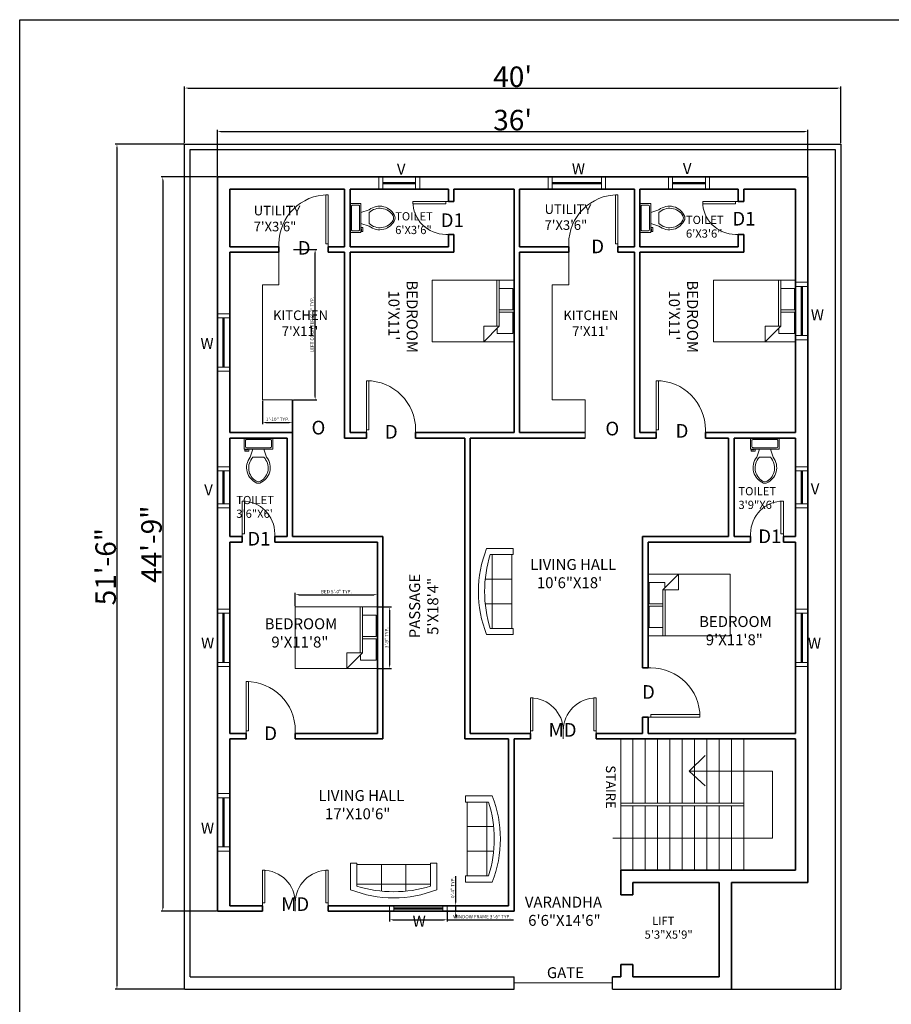
# Model space of a CAD drawing. Units: inches. Extents: x 2169 to 10664, y 1669 to 6352.
# Tile 16 of 17: x 9415 to 10052, y 5632 to 6352. Entities that reach past the tile are written whole.
import ezdxf

# ---------------------------------------------------------------- set-up
doc = ezdxf.new("R2010")
doc.units = ezdxf.units.IN
for name, color, linetype, lineweight in [('A-ANNO-DIMS', 3, 'Continuous', 18), ('A-ANNO-IDEN', 3, 'Continuous', 18), ('A-ANNO-SYMB', 6, 'Continuous', 13), ('A-ANNO-TTLB', 7, 'Continuous', 25), ('A-AREA-IDEN', 4, 'Continuous', 18), ('A-DOOR', 4, 'Continuous', 18), ('A-FLOR-CASE', 8, 'Continuous', 18), ('A-FLOR-FIXT', 9, 'Continuous', 18), ('A-FLOR-STRS', 4, 'Continuous', 18), ('A-FURN', 8, 'Continuous', 18), ('A-GLAZ', 30, 'Continuous', 18), ('A-WALL', 7, 'Continuous', 35), ('C-PROP', 251, 'Continuous', 25)]:
    doc.layers.add(name, color=color, linetype=linetype, lineweight=lineweight)
doc.styles.get("Standard").update_dxf_attribs({"font": 'arial.ttf'})
doc.dimstyles.new('ISO-25', dxfattribs={"dimtxt": 2.5, "dimasz": 2.5, "dimexe": 1.25, "dimexo": 0.625, "dimtad": 1, "dimdec": 0, "dimlunit": 3, "dimtxsty": 'Standard', "dimcen": 2.5, "dimadec": 0, "dimazin": 0, "dimtfac": 1, "dimtdec": 0, "dimtmove": 0, "dimatfit": 3, "dimfxl": 1, "dimarcsym": 0})

# ---------------------------------------------------------------- blocks, each defined once
blk = doc.blocks.new('*U5')
for p, q in [((0, 0), (0, -6)), ((-36, 0), (-36, -6))]:
    blk.add_line(p, q)
blk.add_lwpolyline([(0, 0), (0, 36), (-1.75, 36), (-1.75, 0)], close=True)
blk.add_arc((0, 0), 36, 90, 180)
blk = doc.blocks.new('*U23')
for p, q in [((0, 0), (0, -6)), ((24, 0), (24, -6))]:
    blk.add_line(p, q)
blk.add_lwpolyline([(0, 0), (0, 24), (1.75, 24), (1.75, 0)], close=True)
blk.add_arc((0, 0), 24, 0, 90)
blk = doc.blocks.new('*U22')
for p, q in [((0, 0), (0, -6)), ((36, 0), (36, -6))]:
    blk.add_line(p, q)
blk.add_lwpolyline([(0, 0), (0, 36), (1.75, 36), (1.75, 0)], close=True)
blk.add_arc((0, 0), 36, 0, 90)
blk = doc.blocks.new('*U3')
for p, q in [((-24, 0), (-24, -6)), ((0, 0), (0, -6))]:
    blk.add_line(p, q)
blk.add_lwpolyline([(0, 0), (0, 24), (-1.75, 24), (-1.75, 0)], close=True)
blk.add_arc((0, 0), 24, 90, 180)
blk = doc.blocks.new('*U25')
for p, q in [((0, 0), (0, 6)), ((24, 0), (24, 6))]:
    blk.add_line(p, q)
blk.add_lwpolyline([(0, 0), (0, -24), (1.75, -24), (1.75, 0)], close=True)
blk.add_arc((0, 0), 24, 270, 0)
blk = doc.blocks.new('*U24')
for p, q in [((0, 0), (0, 6)), ((24, 0), (24, 6))]:
    blk.add_line(p, q)
blk.add_lwpolyline([(0, 0), (0, -24), (1.75, -24), (1.75, 0)], close=True)
blk.add_arc((0, 0), 24, 270, 0)
blk = doc.blocks.new('Bed - Queen')
for p, q in [((0, -80.00003), (0, 0)), ((0, 0), (59.99999, 0)), ((59.99999, 0), (59.99999, -80.00003)), ((7.99999, -1.2), (28.79998, -1.2)), ((7.99999, -14.4), (7.99999, -1.2)), ((28.79998, -1.2), (28.79998, -14.4)), ((31.19999, -1.2), (51.99999, -1.2)), ((31.19999, -14.4), (31.19999, -1.2)), ((51.99999, -1.2), (51.99999, -16.4)), ((0, -14.4), (44.8, -14.4)), ((44.8, -16.8), (0, -16.8)), ((59.99999, -29.6), (44.8, -14.4)), ((44.8, -14.4), (44.8, -29.6)), ((51.99999, -16.4), (46.79936, -16.4)), ((44.8, -29.6), (59.99999, -29.6)), ((59.99999, -80.00003), (0, -80.00003))]:
    blk.add_line(p, q)
blk = doc.blocks.new('Sofa - Roundback 7 ft.')
for p, q in [((-12.00002, -32.4421), (-12.00003, -6.5971)), ((11.99997, -32.4421), (11.99998, -6.5971)), ((-36.000027, -34), (-36.000027, -11.4696)), ((-35.999844, -13.3819), (35.9998, -13.3819)), ((35.99998, -34), (35.99998, -11.4696)), ((-36.000027, -32.4421), (35.99998, -32.4421))]:
    blk.add_line(p, q)
for points in [[(-36.000027, -34), (-42.000027, -34), (-42.000027, -8)], [(41.99998, -8), (41.99998, -34), (35.99998, -34)]]:
    blk.add_lwpolyline(points)
for centre, radius, start, end in [((0, -114.25), 114.25, 68.43141, 111.5686), ((-0.00001, -127.1968), 121.1968, 72.72033, 107.2797)]:
    blk.add_arc(centre, radius, start, end)
blk = doc.blocks.new('Toilet - top')
for p, q in [((9.5, -6), (9.5, -2)), ((-10, -8.5), (-8, -8.5)), ((-10, -9.5), (-10, -8.5)), ((-7, -9.5), (-10, -9.5)), ((-8, -8.5), (-8, -8)), ((-7, -8), (-7, -9.5)), ((-4, -8), (-6, -14)), ((4, -14), (-4, -14)), ((4, -8), (6, -14))]:
    blk.add_line(p, q)
blk.add_lwpolyline([(10.5, -8), (10.5, 0), (-10.5, 0), (-10.5, -8)], close=True)
for points in [[(-9.5, -2), (-9.5, -6)], [(8.5, -1), (-8.5, -1)], [(-8.5, -7), (8.5, -7)]]:
    blk.add_lwpolyline(points)
for centre, radius, start, end in [((-8.62, -1.88), 0.884, 81.8699, 188.1301), ((-8.62, -6.12), 0.884, 171.8699, 278.1301), ((8.62, -1.88), 0.884, 351.8699, 98.1301), ((8.62, -6.12), 0.884, 261.8699, 8.1301), ((3.52, -21.58), 12.17, 141.46911, 247.97143), ((4.2, -21.82), 11.33, 136.36773, 238.94682), ((-3.52, -21.58), 12.17, 292.02843, 38.53071), ((-4.2, -21.82), 11.33, 301.05301, 43.63209), ((0, -27.88), 4, 245.73182, 294.26817), ((0, -29), 4, 254.86053, 285.13947)]:
    blk.add_arc(centre, radius, start, end)
blk = doc.blocks.new('*D26')
at = {"layer": 'A-ANNO-DIMS', "color": 0, "lineweight": -2, "transparency": 16777216}
for p, q in [((9559.46, 6237.52), (9559.46, 6271.45)), ((9561.96, 6270.2), (9988.96, 6270.2)), ((9991.46, 6237.52), (9991.46, 6271.45))]:
    blk.add_line(p, q, dxfattribs=at)
at = {"layer": 'A-ANNO-DIMS', "color": 0, "transparency": 16777216}
for points in [[(9561.96, 6270.62), (9561.96, 6269.78), (9559.46, 6270.2)], [(9988.96, 6270.62), (9988.96, 6269.78), (9991.46, 6270.2)]]:
    blk.add_solid(points, dxfattribs=at)
at = {"layer": 'Defpoints', "color": 0, "transparency": 16777216}
for p in [(9991.46, 6270.2), (9559.46, 6236.9), (9991.46, 6236.9)]:
    blk.add_point(p, dxfattribs=at)
at = {"layer": 'A-ANNO-DIMS', "color": 0, "transparency": 16777216, "insert": (9775.46, 6278.49), "char_height": 2.5, "attachment_point": 5}
blk.add_mtext("{\\H6x;36'}", dxfattribs=at)
blk = doc.blocks.new('*D27')
at = {"layer": 'A-ANNO-DIMS', "color": 0, "lineweight": -2, "transparency": 16777216}
for p, q in [((9535.46, 6261.52), (9535.46, 6303.18)), ((9537.96, 6301.93), (10012.96, 6301.93)), ((10015.46, 6261.52), (10015.46, 6303.18))]:
    blk.add_line(p, q, dxfattribs=at)
at = {"layer": 'A-ANNO-DIMS', "color": 0, "transparency": 16777216}
for points in [[(9537.96, 6302.34), (9537.96, 6301.51), (9535.46, 6301.93)], [(10012.96, 6302.34), (10012.96, 6301.51), (10015.46, 6301.93)]]:
    blk.add_solid(points, dxfattribs=at)
at = {"layer": 'Defpoints', "color": 0, "transparency": 16777216}
for p in [(10015.46, 6301.93), (9535.46, 6260.9), (10015.46, 6260.9)]:
    blk.add_point(p, dxfattribs=at)
at = {"layer": 'A-ANNO-DIMS', "color": 0, "transparency": 16777216, "insert": (9775.46, 6310.21), "char_height": 2.5, "attachment_point": 5}
blk.add_mtext("{\\H6x;40'}", dxfattribs=at)
blk = doc.blocks.new('*D28')
at = {"layer": 'A-ANNO-DIMS', "color": 0, "lineweight": -2, "transparency": 16777216}
for p, q in [((9558.84, 6236.9), (9518.24, 6236.9)), ((9519.49, 6234.4), (9519.49, 5702.4)), ((9558.84, 5699.9), (9518.24, 5699.9))]:
    blk.add_line(p, q, dxfattribs=at)
at = {"layer": 'A-ANNO-DIMS', "color": 0, "transparency": 16777216}
for points in [[(9519.08, 6234.4), (9519.91, 6234.4), (9519.49, 6236.9)], [(9519.08, 5702.4), (9519.91, 5702.4), (9519.49, 5699.9)]]:
    blk.add_solid(points, dxfattribs=at)
at = {"layer": 'Defpoints', "color": 0, "transparency": 16777216}
for p in [(9559.46, 6236.9), (9519.49, 5699.9), (9559.46, 5699.9)]:
    blk.add_point(p, dxfattribs=at)
at = {"layer": 'A-ANNO-DIMS', "color": 0, "transparency": 16777216, "insert": (9511.21, 5968.31), "char_height": 2.5, "attachment_point": 5, "rotation": 90}
blk.add_mtext('{\\H6x;44\'-9"}', dxfattribs=at)
blk = doc.blocks.new('*D29')
at = {"layer": 'A-ANNO-DIMS', "color": 0, "lineweight": -2, "transparency": 16777216}
for p, q in [((9534.84, 6260.9), (9484.72, 6260.9)), ((9485.97, 6258.4), (9485.97, 5645.4)), ((9534.84, 5642.9), (9484.72, 5642.9))]:
    blk.add_line(p, q, dxfattribs=at)
at = {"layer": 'A-ANNO-DIMS', "color": 0, "transparency": 16777216}
for points in [[(9485.56, 6258.4), (9486.39, 6258.4), (9485.97, 6260.9)], [(9485.56, 5645.4), (9486.39, 5645.4), (9485.97, 5642.9)]]:
    blk.add_solid(points, dxfattribs=at)
at = {"layer": 'Defpoints', "color": 0, "transparency": 16777216}
for p in [(9535.46, 6260.9), (9485.97, 5642.9), (9535.46, 5642.9)]:
    blk.add_point(p, dxfattribs=at)
at = {"layer": 'A-ANNO-DIMS', "color": 0, "transparency": 16777216, "insert": (9477.69, 5951.9), "char_height": 2.5, "attachment_point": 5, "rotation": 90}
blk.add_mtext('{\\H6x;51\'-6"}', dxfattribs=at)
blk = doc.blocks.new('WIN-36-WALL-9')
for p, q in [((9, 42), (0, 42)), ((9, 39), (0, 39)), ((4, 39), (4, 3)), ((4.5, 39), (4.5, 3)), ((5, 39), (5, 3)), ((9, 3), (0, 3)), ((9, 0), (0, 0))]:
    blk.add_line(p, q)
blk = doc.blocks.new('WIN-24-WALL-9')
for p, q in [((9, 30), (0, 30)), ((9, 27), (0, 27)), ((4, 27), (4, 3)), ((4.5, 27), (4.5, 3)), ((5, 27), (5, 3)), ((9, 3), (0, 3)), ((9, 0), (0, 0))]:
    blk.add_line(p, q)
blk = doc.blocks.new('WIN-36-WALL-4')
for p, q in [((0, 4), (0, 0)), ((3, 4), (3, 0)), ((3, 2.5), (39, 2.5)), ((3, 2), (39, 2)), ((3, 1.5), (39, 1.5)), ((39, 4), (39, 0)), ((42, 4), (42, 0))]:
    blk.add_line(p, q)
blk = doc.blocks.new('STAIR-DOGLEG-PLAN')
for p, q in [((0, 0), (0, 96)), ((9, 49), (9, 96)), ((18, 49), (18, 96)), ((27, 49), (27, 96)), ((36, 49), (36, 96)), ((45, 49), (45, 96)), ((54, 49), (54, 96)), ((63, 49), (63, 96)), ((72, 49), (72, 96)), ((81, 49), (81, 96)), ((90, 0), (90, 96)), ((90, 49), (0, 49)), ((90, 47), (0, 47)), ((9, 0), (9, 47)), ((18, 0), (18, 47)), ((27, 0), (27, 47)), ((36, 0), (36, 47)), ((45, 0), (45, 47)), ((54, 0), (54, 47)), ((63, 0), (63, 47)), ((72, 0), (72, 47)), ((81, 0), (81, 47))]:
    blk.add_line(p, q)
blk = doc.blocks.new('STAIR-DIRECTION')
for p, q in [((55.67, 49), (67.5, 60.35)), ((116.68, 49), (55.67, 49)), ((55.67, 49), (67.5, 38.08)), ((116.68, 0), (116.68, 49)), ((0, 0), (116.68, 0))]:
    blk.add_line(p, q)
blk = doc.blocks.new('COUNTER-UTILITY-L')
for p, q in [((12, 110), (12, 84)), ((0, 0), (0, 84)), ((0, 84), (12, 84)), ((0, 0), (22, 0))]:
    blk.add_line(p, q)
blk = doc.blocks.new('COUNTER-UTILITY-R')
for p, q in [((12, 136), (12, 112)), ((0, 28), (0, 112)), ((0, 112), (12, 112)), ((0, 28), (24, 28)), ((24, 0), (24, 28))]:
    blk.add_line(p, q)
blk = doc.blocks.new('*D55')
at = {"layer": 'A-ANNO-DIMS', "color": 0, "lineweight": -2, "transparency": 16777216}
for p, q in [((9616.46, 5923.02), (9616.46, 5932.65)), ((9618.96, 5931.4), (9673.96, 5931.4)), ((9676.46, 5923.02), (9676.46, 5932.65))]:
    blk.add_line(p, q, dxfattribs=at)
at = {"layer": 'A-ANNO-DIMS', "color": 0, "transparency": 16777216}
for points in [[(9618.96, 5931.81), (9618.96, 5930.98), (9616.46, 5931.4)], [(9673.96, 5931.81), (9673.96, 5930.98), (9676.46, 5931.4)]]:
    blk.add_solid(points, dxfattribs=at)
at = {"layer": 'Defpoints', "color": 0, "transparency": 16777216}
for p in [(9676.46, 5931.4), (9616.46, 5922.4), (9676.46, 5922.4)]:
    blk.add_point(p, dxfattribs=at)
at = {"layer": 'A-ANNO-DIMS', "color": 0, "transparency": 16777216, "insert": (9646.46, 5933.3), "char_height": 2.5, "attachment_point": 5}
blk.add_mtext('BED 5\'-0" TYP.', dxfattribs=at)
blk = doc.blocks.new('*D56')
at = {"layer": 'A-ANNO-DIMS', "color": 0, "lineweight": -2, "transparency": 16777216}
for p, q in [((9677.09, 5922.4), (9686.71, 5922.4)), ((9685.46, 5919.9), (9685.46, 5879.9)), ((9677.09, 5877.4), (9686.71, 5877.4))]:
    blk.add_line(p, q, dxfattribs=at)
at = {"layer": 'A-ANNO-DIMS', "color": 0, "transparency": 16777216}
for points in [[(9685.05, 5919.9), (9685.88, 5919.9), (9685.46, 5922.4)], [(9685.05, 5879.9), (9685.88, 5879.9), (9685.46, 5877.4)]]:
    blk.add_solid(points, dxfattribs=at)
at = {"layer": 'Defpoints', "color": 0, "transparency": 16777216}
for p in [(9676.46, 5922.4), (9676.46, 5877.4), (9685.46, 5877.4)]:
    blk.add_point(p, dxfattribs=at)
at = {"layer": 'A-ANNO-DIMS', "color": 0, "transparency": 16777216, "insert": (9683.56, 5899.9), "char_height": 2.5, "attachment_point": 5, "rotation": 90}
blk.add_mtext('3\'-9" TYP.', dxfattribs=at)
blk = doc.blocks.new('*D75')
at = {"layer": 'A-ANNO-DIMS', "color": 0, "lineweight": -2, "transparency": 16777216}
for p, q in [((9685.46, 5699.27), (9685.46, 5692.35)), ((9727.46, 5699.27), (9727.46, 5692.35)), ((9687.96, 5693.6), (9724.96, 5693.6)), ((9727.46, 5693.6), (9776.04, 5693.6))]:
    blk.add_line(p, q, dxfattribs=at)
at = {"layer": 'A-ANNO-DIMS', "color": 0, "transparency": 16777216}
for points in [[(9687.96, 5694.01), (9687.96, 5693.18), (9685.46, 5693.6)], [(9724.96, 5694.01), (9724.96, 5693.18), (9727.46, 5693.6)]]:
    blk.add_solid(points, dxfattribs=at)
at = {"layer": 'Defpoints', "color": 0, "transparency": 16777216}
for p in [(9685.46, 5699.9), (9727.46, 5699.9), (9727.46, 5693.6)]:
    blk.add_point(p, dxfattribs=at)
at = {"layer": 'A-ANNO-DIMS', "color": 0, "transparency": 16777216, "insert": (9753, 5695.52), "char_height": 2.5, "attachment_point": 5}
blk.add_mtext('WINDOW FRAME 3\'-6" TYP.', dxfattribs=at)
blk = doc.blocks.new('*D76')
at = {"layer": 'A-ANNO-DIMS', "color": 0, "lineweight": -2, "transparency": 16777216}
for p, q in [((9733.76, 5706.4), (9733.76, 5725.39)), ((9728.09, 5703.9), (9735.01, 5703.9)), ((9733.76, 5699.9), (9733.76, 5703.9)), ((9728.09, 5699.9), (9735.01, 5699.9)), ((9733.76, 5697.4), (9733.76, 5694.9))]:
    blk.add_line(p, q, dxfattribs=at)
at = {"layer": 'A-ANNO-DIMS', "color": 0, "transparency": 16777216}
for points in [[(9733.35, 5706.4), (9734.18, 5706.4), (9733.76, 5703.9)], [(9733.35, 5697.4), (9734.18, 5697.4), (9733.76, 5699.9)]]:
    blk.add_solid(points, dxfattribs=at)
at = {"layer": 'Defpoints', "color": 0, "transparency": 16777216}
for p in [(9727.46, 5703.9), (9733.76, 5703.9), (9727.46, 5699.9)]:
    blk.add_point(p, dxfattribs=at)
at = {"layer": 'A-ANNO-DIMS', "color": 0, "transparency": 16777216, "insert": (9731.86, 5717.14), "char_height": 2.5, "attachment_point": 5, "rotation": 90}
blk.add_mtext('0\'-4" TYP.', dxfattribs=at)
blk = doc.blocks.new('*D81')
at = {"layer": 'A-ANNO-DIMS', "color": 0, "lineweight": -2, "transparency": 16777216}
for p, q in [((9615.09, 6183.9), (9632.21, 6183.9)), ((9630.96, 6076.4), (9630.96, 6181.4)), ((9615.09, 6073.9), (9632.21, 6073.9))]:
    blk.add_line(p, q, dxfattribs=at)
at = {"layer": 'A-ANNO-DIMS', "color": 0, "transparency": 16777216}
for points in [[(9630.55, 6181.4), (9631.38, 6181.4), (9630.96, 6183.9)], [(9630.55, 6076.4), (9631.38, 6076.4), (9630.96, 6073.9)]]:
    blk.add_solid(points, dxfattribs=at)
at = {"layer": 'Defpoints', "color": 0, "transparency": 16777216}
for p in [(9614.46, 6183.9), (9630.96, 6183.9), (9614.46, 6073.9)]:
    blk.add_point(p, dxfattribs=at)
at = {"layer": 'A-ANNO-DIMS', "color": 0, "transparency": 16777216, "insert": (9629.04, 6128.9), "char_height": 2.5, "attachment_point": 5, "rotation": 90}
blk.add_mtext('LEFT COUNTER 9\'-2" TYP.', dxfattribs=at)
blk = doc.blocks.new('*D82')
at = {"layer": 'A-ANNO-DIMS', "color": 0, "lineweight": -2, "transparency": 16777216}
for p, q in [((9592.46, 6073.27), (9592.46, 6056.15)), ((9614.46, 6073.27), (9614.46, 6056.15)), ((9594.96, 6057.4), (9611.96, 6057.4))]:
    blk.add_line(p, q, dxfattribs=at)
at = {"layer": 'A-ANNO-DIMS', "color": 0, "transparency": 16777216}
for points in [[(9594.96, 6057.81), (9594.96, 6056.98), (9592.46, 6057.4)], [(9611.96, 6057.81), (9611.96, 6056.98), (9614.46, 6057.4)]]:
    blk.add_solid(points, dxfattribs=at)
at = {"layer": 'Defpoints', "color": 0, "transparency": 16777216}
for p in [(9592.46, 6073.9), (9614.46, 6073.9), (9614.46, 6057.4)]:
    blk.add_point(p, dxfattribs=at)
at = {"layer": 'A-ANNO-DIMS', "color": 0, "transparency": 16777216, "insert": (9603.46, 6059.3), "char_height": 2.5, "attachment_point": 5}
blk.add_mtext('1\'-10" TYP.', dxfattribs=at)

msp = doc.modelspace()

# ---------------------------------------------------------------- linework, layer by layer
at = {"layer": 'A-ANNO-TTLB'}
msp.add_lwpolyline([(9414.82, 6351.94), (10664.28, 6351.94), (10664.28, 5158.92), (9414.82, 5158.92)], close=True, dxfattribs=at)
at = {"layer": 'A-DOOR'}
msp.add_line((9776.46, 5647.4), (9848.46, 5647.4), dxfattribs=at)
at = {"layer": 'A-WALL'}
for p, q in [((9559.46, 6236.9), (9991.46, 6236.9)), ((9559.46, 5699.9), (9559.46, 6236.9)), ((9991.46, 6236.9), (9991.46, 5720.9)), ((9568.46, 6227.9), (9652.46, 6227.9)), ((9568.46, 6185.9), (9568.46, 6227.9)), ((9652.46, 6185.9), (9652.46, 6227.9)), ((9656.46, 6227.9), (9728.46, 6227.9)), ((9656.46, 6185.9), (9656.46, 6227.9)), ((9728.46, 6218.9), (9728.46, 6227.9)), ((9732.46, 6227.9), (9776.46, 6227.9)), ((9732.46, 6218.9), (9732.46, 6227.9)), ((9776.46, 6049.9), (9776.46, 6227.9)), ((9780.46, 6227.9), (9864.46, 6227.9)), ((9780.46, 6185.9), (9780.46, 6227.9)), ((9864.46, 6185.9), (9864.46, 6227.9)), ((9868.46, 6227.9), (9940.46, 6227.9)), ((9868.46, 6185.9), (9868.46, 6227.9)), ((9940.46, 6218.9), (9940.46, 6227.9)), ((9944.46, 6227.9), (9982.46, 6227.9)), ((9944.46, 6218.9), (9944.46, 6227.9)), ((9982.46, 6227.9), (9982.46, 6049.9)), ((9728.46, 6218.9), (9732.46, 6218.9)), ((9940.46, 6218.9), (9944.46, 6218.9)), ((9728.46, 6185.9), (9728.46, 6194.9)), ((9728.46, 6194.9), (9732.46, 6194.9)), ((9732.46, 6181.9), (9732.46, 6194.9)), ((9940.46, 6185.9), (9940.46, 6194.9)), ((9940.46, 6194.9), (9944.46, 6194.9)), ((9944.46, 6181.9), (9944.46, 6194.9)), ((9568.46, 6185.9), (9604.46, 6185.9)), ((9568.46, 6181.9), (9604.46, 6181.9)), ((9568.46, 6049.9), (9568.46, 6181.9)), ((9604.46, 6181.9), (9604.46, 6185.9)), ((9640.46, 6185.9), (9652.46, 6185.9)), ((9640.46, 6181.9), (9640.46, 6185.9)), ((9640.46, 6181.9), (9652.46, 6181.9)), ((9652.46, 6045.9), (9652.46, 6181.9)), ((9656.46, 6185.9), (9728.46, 6185.9)), ((9656.46, 6181.9), (9732.46, 6181.9)), ((9656.46, 6049.9), (9656.46, 6181.9)), ((9780.46, 6185.9), (9816.46, 6185.9)), ((9780.46, 6181.9), (9816.46, 6181.9)), ((9780.46, 6049.9), (9780.46, 6181.9)), ((9816.46, 6181.9), (9816.46, 6185.9)), ((9852.46, 6185.9), (9864.46, 6185.9)), ((9852.46, 6181.9), (9852.46, 6185.9)), ((9852.46, 6181.9), (9864.46, 6181.9)), ((9864.46, 6045.9), (9864.46, 6181.9)), ((9868.46, 6185.9), (9940.46, 6185.9)), ((9868.46, 6181.9), (9944.46, 6181.9)), ((9868.46, 6049.9), (9868.46, 6181.9)), ((9614.46, 5973.9), (9614.46, 6073.9)), ((9568.46, 6049.9), (9614.46, 6049.9)), ((9656.46, 6049.9), (9668.46, 6049.9)), ((9668.46, 6045.9), (9668.46, 6049.9)), ((9704.46, 6049.9), (9776.46, 6049.9)), ((9704.46, 6045.9), (9704.46, 6049.9)), ((9780.46, 6049.9), (9828.46, 6049.9)), ((9868.46, 6049.9), (9880.46, 6049.9)), ((9880.46, 6045.9), (9880.46, 6049.9)), ((9916.46, 6049.9), (9982.46, 6049.9)), ((9916.46, 6045.9), (9916.46, 6049.9)), ((9568.46, 6045.9), (9610.46, 6045.9)), ((9568.46, 5973.9), (9568.46, 6045.9)), ((9610.46, 5973.9), (9610.46, 6045.9)), ((9652.46, 6045.9), (9668.46, 6045.9)), ((9704.46, 6045.9), (9740.46, 6045.9)), ((9740.46, 5825.9), (9740.46, 6045.9)), ((9744.46, 6045.9), (9828.46, 6045.9)), ((9744.46, 5829.9), (9744.46, 6045.9)), ((9864.46, 6045.9), (9880.46, 6045.9)), ((9916.46, 6045.9), (9933.46, 6045.9)), ((9933.46, 6045.9), (9933.46, 5973.9)), ((9937.46, 6045.9), (9982.46, 6045.9)), ((9937.46, 6045.9), (9937.46, 5973.9)), ((9982.46, 6045.9), (9982.46, 5973.9)), ((9568.46, 5973.9), (9577.46, 5973.9)), ((9577.46, 5969.9), (9577.46, 5973.9)), ((9601.46, 5973.9), (9610.46, 5973.9)), ((9601.46, 5969.9), (9601.46, 5973.9)), ((9614.46, 5973.9), (9680.46, 5973.9)), ((9680.46, 5825.9), (9680.46, 5973.9)), ((9870.46, 5973.9), (9933.46, 5973.9)), ((9870.46, 5973.9), (9870.46, 5877.9)), ((9937.46, 5973.9), (9949.46, 5973.9)), ((9949.46, 5973.9), (9949.46, 5969.9)), ((9973.46, 5973.9), (9982.46, 5973.9)), ((9973.46, 5973.9), (9973.46, 5969.9)), ((9568.46, 5969.9), (9577.46, 5969.9)), ((9568.46, 5829.9), (9568.46, 5969.9)), ((9601.46, 5969.9), (9676.46, 5969.9)), ((9676.46, 5829.9), (9676.46, 5969.9)), ((9874.46, 5969.9), (9949.46, 5969.9)), ((9874.46, 5969.9), (9874.46, 5877.9)), ((9973.46, 5969.9), (9982.46, 5969.9)), ((9982.46, 5969.9), (9982.46, 5829.9)), ((9870.46, 5877.9), (9874.46, 5877.9)), ((9870.46, 5841.9), (9874.46, 5841.9)), ((9870.46, 5841.9), (9870.46, 5829.9)), ((9874.46, 5841.9), (9874.46, 5829.9)), ((9568.46, 5829.9), (9580.46, 5829.9)), ((9580.46, 5825.9), (9580.46, 5829.9)), ((9616.46, 5829.9), (9676.46, 5829.9)), ((9616.46, 5825.9), (9616.46, 5829.9)), ((9744.46, 5829.9), (9788.46, 5829.9)), ((9788.46, 5825.9), (9788.46, 5829.9)), ((9836.46, 5829.9), (9870.46, 5829.9)), ((9836.46, 5825.9), (9836.46, 5829.9)), ((9874.46, 5829.9), (9982.46, 5829.9)), ((9568.46, 5825.9), (9580.46, 5825.9)), ((9568.46, 5703.9), (9568.46, 5825.9)), ((9616.46, 5825.9), (9680.46, 5825.9)), ((9740.46, 5825.9), (9772.46, 5825.9)), ((9772.46, 5703.9), (9772.46, 5825.9)), ((9776.46, 5825.9), (9788.46, 5825.9)), ((9776.46, 5699.9), (9776.46, 5825.9)), ((9836.46, 5825.9), (9982.46, 5825.9)), ((9982.46, 5825.9), (9982.46, 5729.9)), ((9982.46, 5729.9), (9854.46, 5729.9)), ((9854.46, 5711.9), (9854.46, 5729.9)), ((9926.46, 5720.9), (9863.46, 5720.9)), ((9863.46, 5711.9), (9863.46, 5720.9)), ((9926.46, 5651.9), (9926.46, 5720.9)), ((9991.46, 5720.9), (9935.46, 5720.9)), ((9935.46, 5642.9), (9935.46, 5720.9)), ((9863.46, 5711.9), (9854.46, 5711.9)), ((9592.46, 5703.9), (9568.46, 5703.9)), ((9592.46, 5699.9), (9592.46, 5703.9)), ((9772.46, 5703.9), (9640.46, 5703.9)), ((9640.46, 5699.9), (9640.46, 5703.9)), ((9592.46, 5699.9), (9559.46, 5699.9)), ((9776.46, 5699.9), (9640.46, 5699.9)), ((9854.46, 5651.9), (9854.46, 5660.9)), ((9854.46, 5660.9), (9863.46, 5660.9)), ((9863.46, 5651.9), (9863.46, 5660.9)), ((9848.46, 5651.9), (9854.46, 5651.9)), ((9863.46, 5651.9), (9926.46, 5651.9))]:
    msp.add_line(p, q, dxfattribs=at)
at = {"layer": 'C-PROP'}
for p, q in [((9535.46, 6260.9), (10015.46, 6260.9)), ((9535.46, 5642.9), (9535.46, 6260.9)), ((10015.46, 6260.9), (10015.46, 5642.9)), ((9539.46, 6256.9), (10011.46, 6256.9)), ((9539.46, 5651.9), (9539.46, 6256.9)), ((10011.46, 6256.9), (10011.46, 5642.9)), ((9539.46, 5651.9), (9776.46, 5651.9)), ((9776.46, 5642.9), (9776.46, 5651.9)), ((9848.46, 5642.9), (9848.46, 5651.9)), ((9535.46, 5642.9), (9776.46, 5642.9)), ((9848.46, 5642.9), (9935.46, 5642.9)), ((9935.46, 5642.9), (10015.46, 5642.9))]:
    msp.add_line(p, q, dxfattribs=at)

# ---------------------------------------------------------------- block references
at = {"layer": 'A-ANNO-SYMB'}
msp.add_blockref('STAIR-DIRECTION', (9848.79, 5753.4), dxfattribs=at)
at = {"layer": 'A-DOOR'}
for name, p in [('*U5', (9640.46, 6187.9)), ('*U5', (9852.46, 6187.9)), ('*U22', (9668.46, 6051.9)), ('*U22', (9880.46, 6051.9)), ('*U23', (9577.46, 5975.9)), ('*U3', (9973.46, 5975.9)), ('*U22', (9580.46, 5831.9)), ('*U23', (9788.46, 5831.9)), ('*U3', (9836.46, 5831.9)), ('*U23', (9592.46, 5705.9)), ('*U3', (9640.46, 5705.9))]:
    msp.add_blockref(name, p, dxfattribs=at)
at = {"layer": 'A-DOOR', "rotation": 270}
for name, p in [('*U24', (9726.46, 6218.9)), ('*U25', (9938.46, 6218.9)), ('*U5', (9876.46, 5841.9))]:
    msp.add_blockref(name, p, dxfattribs=at)
at = {"layer": 'A-FLOR-CASE'}
for name, p in [('COUNTER-UTILITY-L', (9592.46, 6073.9)), ('COUNTER-UTILITY-R', (9804.46, 6045.9))]:
    msp.add_blockref(name, p, dxfattribs=at)
at = {"layer": 'A-FLOR-FIXT', "rotation": 90}
for p in [(9656.46, 6206.9), (9868.46, 6206.9)]:
    msp.add_blockref('Toilet - top', p, dxfattribs=at)
at = {"layer": 'A-FLOR-FIXT'}
for p in [(9589.46, 6045.9), (9959.96, 6045.9)]:
    msp.add_blockref('Toilet - top', p, dxfattribs=at)
at = {"layer": 'A-FLOR-STRS'}
msp.add_blockref('STAIR-DOGLEG-PLAN', (9854.46, 5729.9), dxfattribs=at)
at = {"layer": 'A-FURN', "xscale": 0.75, "yscale": 0.75, "zscale": 0.75}
for name, p, rotation in [('Bed - Queen', (9776.46, 6161.4), 270), ('Bed - Queen', (9982.46, 6161.4), 270), ('Sofa - Roundback 7 ft.', (9750.42, 5933.68), 89.99999999999999), ('Bed - Queen', (9874.46, 5901.4), 89.99999999999999), ('Bed - Queen', (9676.46, 5922.4), 270), ('Sofa - Roundback 7 ft.', (9766.49, 5752.74), 270), ('Sofa - Roundback 7 ft.', (9688.42, 5709.62), 180)]:
    msp.add_blockref(name, p, dxfattribs=dict(at, rotation=rotation))
at = {"layer": 'A-GLAZ'}
for name, p, rotation in [('WIN-24-WALL-9', (9707.46, 6227.9), 89.9999999999965), ('WIN-36-WALL-9', (9801.46, 6236.9), 269.9999999999998), ('WIN-24-WALL-9', (9889.46, 6236.9), 270.0000000000003), ('WIN-24-WALL-9', (9568.46, 6024.9), 180), ('WIN-24-WALL-9', (9991.46, 6024.9), 180)]:
    msp.add_blockref(name, p, dxfattribs=dict(at, rotation=rotation))
for name, p in [('WIN-36-WALL-9', (9982.46, 6117.9)), ('WIN-36-WALL-9', (9559.46, 6094.9)), ('WIN-36-WALL-9', (9559.46, 5878.9)), ('WIN-36-WALL-9', (9982.46, 5878.9)), ('WIN-36-WALL-9', (9559.46, 5743.9)), ('WIN-36-WALL-4', (9685.46, 5699.9))]:
    msp.add_blockref(name, p, dxfattribs=at)

# ---------------------------------------------------------------- texts
at = {"layer": 'A-ANNO-IDEN', "attachment_point": 1}
for s, heights, insert, char_height in [('V', [8.65], (9690.78, 6246.71), 8), ('W', [8.65], (9818.77, 6246.94), 8), ('V', [8.65], (9900, 6247.05), 8), ('D1', [0], (9722.82, 6210.27), 10), ('D1', [0], (9936.16, 6211.38), 10), ('D', [0], (9618.17, 6190.08), 10), ('D', [0], (9832.93, 6191.13), 10), ('W', [8.65], (9993.59, 6140.13), 8), ('W', [8.65], (9547.09, 6119.19), 8), ('O', [8.65], (9628.3, 6058.58), 10), ('O', [8.65], (9843.27, 6057.89), 10), ('D', [0], (9681.96, 6055.52), 10), ('D', [0], (9894.64, 6056.19), 10), ('V', [8.65], (9549.81, 6012.07), 8), ('V', [8.65], (9993.53, 6012.74), 8), ('D1', [0], (9581.35, 5977.32), 10), ('D1', [0], (9955.12, 5979.07), 10), ('W', [8.65], (9547.52, 5900.03), 8), ('W', [8.65], (9991.46, 5899.85), 8), ('D', [0], (9870.07, 5865.22), 10), ('D', [0], (9593.71, 5834.99), 10), ('MD', [8.65], (9801.72, 5837.48), 10), ('W', [8.65], (9547.43, 5764.66), 8), ('MD', [8.65], (9606.12, 5710.07), 10), ('W', [8.65], (9702.27, 5696.56), 8)]:
    msp.add_mtext_dynamic_manual_height_columns(s, width=418.9353, gutter_width=12.5, heights=heights, dxfattribs=dict(at, insert=insert, char_height=char_height))
at = {"layer": 'A-AREA-IDEN', "attachment_point": 1}
for s, width, insert, char_height in [('UTILITY\\P7\'X3\'6"', 378.2909, (9586, 6215.8), 7), ('UTILITY\\P7\'X3\'6"', 378.2909, (9798.79, 6216.87), 7), ('TOILET\\P6\'X3\'6"', 229.0681, (9689.5, 6211.14), 6), ('TOILET\\P6\'X3\'6"', 229.0681, (9902.22, 6208.52), 6), ("KITCHEN\\P   7'X11'", 624.2169, (9600.12, 6139.26), 7), ("KITCHEN\\P   7'X11'", 624.2169, (9812.57, 6139.23), 7), ('TOILET\\P3\'9"X6\'', 181.098, (9940.61, 6010.09), 6), ('TOILET\\P3\'6"X6\'', 181.098, (9573.29, 6003.61), 6), ('LIVING HALL\\P  10\'6"X18\'', 560.0068, (9788.29, 5957.48), 8), ('BEDROOM\\P  9\'X11\'8"', 585.4842, (9594.05, 5914.09), 8), ('BEDROOM\\P  9\'X11\'8"', 585.4842, (9911.86, 5915.74), 8), ('LIVING HALL\\P  17\'X10\'6"', 430.6105, (9633.29, 5788.47), 8), ('VARANDHA\\P 6\'6"X14\'6"', 244.2229, (9784.37, 5710.52), 8), ('   LIFT\\P5\'3"X5\'9"', 367.579, (9871.98, 5695.77), 6), ('GATE', 121.9604, (9800.51, 5658.92), 8)]:
    msp.add_mtext_dynamic_manual_height_columns(s, width=width, gutter_width=12.5, heights=[0], dxfattribs=dict(at, insert=insert, char_height=char_height))
for s, width, insert, char_height, rotation in [("BEDROOM\\P   10'X11'", 613.8035, (9705.93, 6161.25), 8, 270), ("BEDROOM\\P   10'X11'", 613.8035, (9911.06, 6161.25), 8, 270), ('PASSAGE\\P 5\'X18\'4"', 733.7273, (9699.75, 5899.53), 8, 90), ('STAIRE', 319.0814, (9850.7, 5806.57), 7, 270)]:
    msp.add_mtext_dynamic_manual_height_columns(s, width=width, gutter_width=12.5, heights=[0], dxfattribs=dict(at, insert=insert, char_height=char_height, rotation=rotation))

# ---------------------------------------------------------------- dimensions: what is measured, and where the dimension line sits
at = {"layer": 'A-ANNO-DIMS'}
for base, p1, p2, text, override, picture, middle in [((10015.46, 6301.93), (9535.46, 6260.9), (10015.46, 6260.9), '{\\H6x;<>}', {"dimclrd": 0, "dimclre": 0, "dimclrt": 0}, '*D27', (9775.46, 6310.21)), ((9614.46, 6057.4), (9592.46, 6073.9), (9614.46, 6073.9), '<> TYP.', {"dimdec": 1, "dimlfac": 1, "dimrnd": 0, "dimzin": 1, "dimdsep": 46, "dimlunit": 4, "dimfrac": 2}, '*D82', (9603.46, 6059.3)), ((9676.46, 5931.4), (9616.46, 5922.4), (9676.46, 5922.4), 'BED <> TYP.', {"dimdec": 1, "dimlfac": 1, "dimrnd": 0, "dimzin": 1, "dimdsep": 46, "dimlunit": 4, "dimfrac": 2}, '*D55', (9646.46, 5933.3)), ((9727.46, 5693.6), (9685.46, 5699.9), (9727.46, 5699.9), 'WINDOW FRAME <> TYP.', {"dimdec": 1, "dimlfac": 1, "dimrnd": 0, "dimzin": 1, "dimdsep": 46, "dimlunit": 4, "dimfrac": 2}, '*D75', (9753, 5695.52))]:
    dim = msp.add_linear_dim(base=base, p1=p1, p2=p2, text=text, dimstyle='ISO-25', override=override, dxfattribs=at)
    dim.commit()
    dim.dimension.update_dxf_attribs({"geometry": picture, "text_midpoint": middle})
dim = msp.add_linear_dim(base=(9991.46, 6270.2), p1=(9559.46, 6236.9), p2=(9991.46, 6236.9), text='{\\H6x;<>}', dimstyle='ISO-25', override={"dimclrd": 0, "dimclre": 0, "dimclrt": 0}, dxfattribs=at)
dim.commit()
dim.dimension.update_dxf_attribs({"geometry": '*D26', "text_midpoint": (9775.46, 6270.2), "dimtype": 160})
for base, p1, p2, picture, middle in [((9485.97, 5642.9), (9535.46, 6260.9), (9535.46, 5642.9), '*D29', (9485.97, 5951.9)), ((9519.49, 5699.9), (9559.46, 6236.9), (9559.46, 5699.9), '*D28', (9519.49, 5968.31))]:
    dim = msp.add_linear_dim(base=base, p1=p1, p2=p2, angle=90, text='{\\H6x;<>}', dimstyle='ISO-25', override={"dimclrd": 0, "dimclre": 0, "dimclrt": 0}, dxfattribs=at)
    dim.commit()
    dim.dimension.update_dxf_attribs({"geometry": picture, "text_midpoint": middle, "dimtype": 160})
for base, p1, p2, angle, text, picture, middle in [((9630.96, 6183.9), (9614.46, 6073.9), (9614.46, 6183.9), 90, 'LEFT COUNTER <> TYP.', '*D81', (9629.04, 6128.9)), ((9685.46, 5877.4), (9676.46, 5922.4), (9676.46, 5877.4), 270, '<> TYP.', '*D56', (9683.56, 5899.9)), ((9733.76, 5703.9), (9727.46, 5699.9), (9727.46, 5703.9), 90, '<> TYP.', '*D76', (9731.86, 5717.14))]:
    dim = msp.add_linear_dim(base=base, p1=p1, p2=p2, angle=angle, text=text, dimstyle='ISO-25', override={"dimdec": 1, "dimlfac": 1, "dimrnd": 0, "dimzin": 1, "dimdsep": 46, "dimlunit": 4, "dimfrac": 2}, dxfattribs=at)
    dim.commit()
    dim.dimension.update_dxf_attribs({"geometry": picture, "text_midpoint": middle})

doc.saveas('drawing.dxf')
